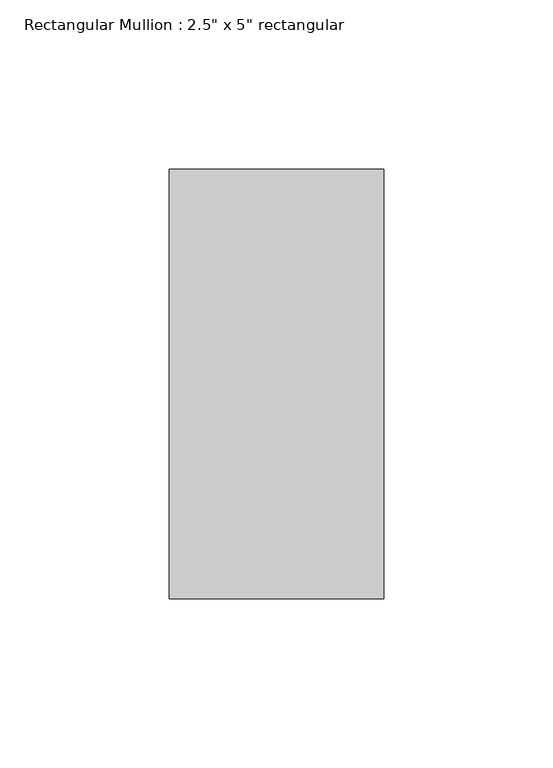
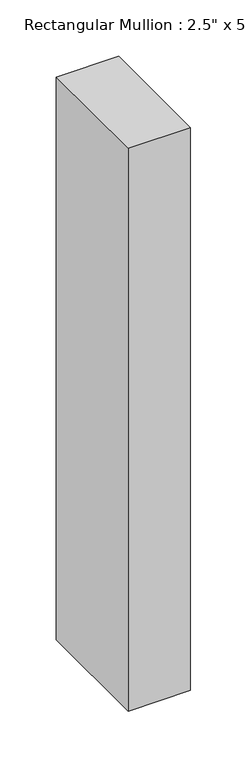
"""IFC4 building model written with IfcOpenShell, lengths in millimetres: member geometry."""

from ifc_helpers import new_model, si_unit, frame, origin, place, context, project, spatial, polyline, outline, extrude, source, transform, mapped, element, save


def member_589dede6(model_context):
    return source(origin(), model_context, "Body", "SweptSolid", [
        extrude(outline(polyline([(0.0, 63.5), (0.0, -63.5), (-63.5, -63.5), (-63.5, 63.5), (0.0, 63.5)])), frame((0.0, 0.0, -609.1997047), z_axis=(0.0, 0.0, 1.0), x_axis=(1.0, 0.0, 0.0)), (0.0, 0.0, 1.0), 609.1997047),
    ])


if __name__ == "__main__":
    model = new_model("IFC4")
    model_context = context("Model", 3, world=origin())
    ifc_project = project(units=[si_unit("LENGTHUNIT", "METRE", prefix="MILLI")], contexts=[model_context])
    site = spatial("IfcSite", under=ifc_project)
    building = spatial("IfcBuilding", under=site)
    placement = place(None, origin())
    member_shape = member_589dede6(model_context)
    element("IfcMember", 1, ObjectType="Rectangular Mullion : 2.5\" x 5\" rectangular", at=placement, inside=building, context=model_context, shape_type="MappedRepresentation", body=[
        mapped(member_shape, transform((0.0, 0.0, 0.0), x_axis=(1.0, 0.0, 0.0), y_axis=(0.0, 1.0, 0.0), z_axis=(0.0, 0.0, 1.0))),
    ])
    save(model, "model.ifc")

# Revit data of these elements
# Type "Rectangular Mullion : 2.5\" x 5\" rectangular"
#   built-in parameter 1007304 = 0.416667 (stored number, unit not read)
#   built-in parameter 1007301 = 0.104167 (stored number, unit not read)
#   built-in parameter 1007300 = 0.104167 (stored number, unit not read)
# Element 1 (IfcMember, "Rectangular Mullion : 2.5\" x 5\" rectangular")
#   Materials on its faces: "Aluminum"
# Materials
#   "Aluminum": class "Metal", colour RGB 247 247 247, transparency 0, Description = "Aluminum 6061", Cost = 0
